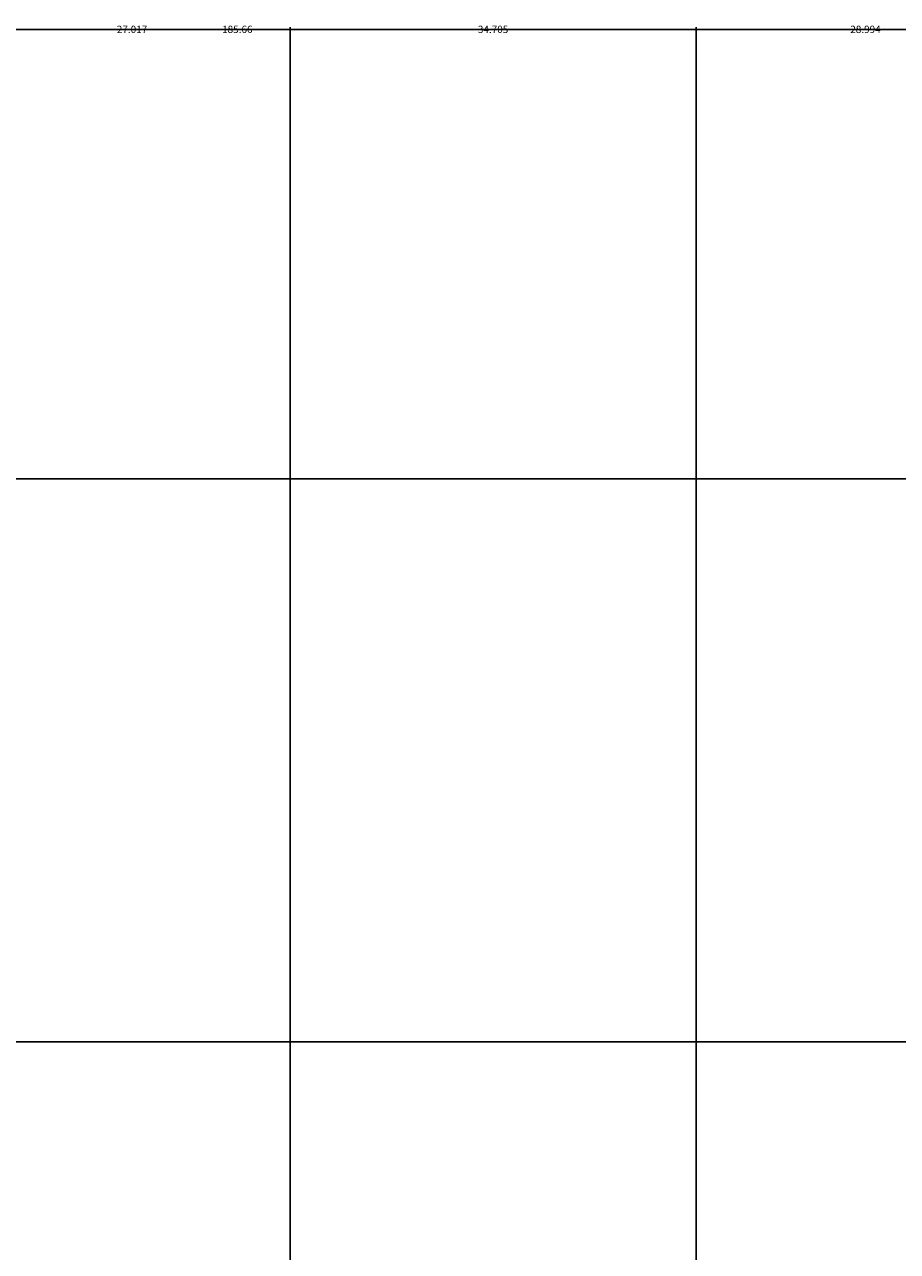
# Model space of a CAD drawing. Units: inches. Extents: x -13 to 809, y 112 to 656.
# Tile 32 of 55: x 182 to 257, y 551 to 656. Entities that reach past the tile are written whole.
import ezdxf

# ---------------------------------------------------------------- set-up
doc = ezdxf.new("R2010")
doc.units = ezdxf.units.IN
doc.header["$MEASUREMENT"] = 0
doc.layers.add('A-ANNO-DIMS', color=2, linetype='Continuous', lineweight=18)
doc.styles.get("Standard").update_dxf_attribs({"font": 'arial.ttf'})
doc.dimstyles.get("Standard").update_dxf_attribs({"dimtxt": 0.625, "dimasz": 0.18, "dimexe": 0.18, "dimexo": 0.0625, "dimgap": 0.09, "dimtad": 0, "dimtih": 1, "dimtoh": 1, "dimdec": 4, "dimzin": 0, "dimdsep": 46, "dimlunit": 4, "dimtxsty": 'Standard', "dimcen": 0.09, "dimadec": 0, "dimazin": 0, "dimtfac": 1, "dimtdec": 4, "dimtofl": 0, "dimtmove": 0, "dimatfit": 3, "dimfxl": 1, "dimtolj": 1, "dimtzin": 0, "dimarcsym": 0})

# ---------------------------------------------------------------- blocks, each defined once
blk = doc.blocks.new('*D23')
at = {"layer": 'A-ANNO-DIMS', "color": 0, "lineweight": -2, "transparency": 16777216}
for p, q in [((107.26, 510.58), (107.26, 655.96)), ((107.44, 655.78), (198.73, 655.78)), ((292.74, 655.78), (201.45, 655.78)), ((292.92, 569.3), (292.92, 655.96))]:
    blk.add_line(p, q, dxfattribs=at)
at = {"layer": 'A-ANNO-DIMS', "color": 0, "transparency": 16777216}
for points in [[(107.44, 655.81), (107.44, 655.75), (107.26, 655.78)], [(292.74, 655.81), (292.74, 655.75), (292.92, 655.78)]]:
    blk.add_solid(points, dxfattribs=at)
at = {"layer": 'Defpoints', "color": 0, "transparency": 16777216}
for p in [(292.92, 655.78), (292.92, 569.24), (107.26, 510.52)]:
    blk.add_point(p, dxfattribs=at)
at = {"layer": 'A-ANNO-DIMS', "color": 0, "transparency": 16777216, "insert": (200.09, 655.78), "char_height": 0.625, "attachment_point": 5}
blk.add_mtext('\\A1;185.66', dxfattribs=at)
blk = doc.blocks.new('*D36')
at = {"layer": 'A-ANNO-DIMS', "color": 0, "lineweight": -2, "transparency": 16777216}
for p, q in [((311.64, 569.24), (-12.1, 569.24)), ((-11.92, 569.06), (-11.92, 540.29)), ((-11.92, 510.7), (-11.92, 539.47)), ((107.2, 510.52), (-12.1, 510.52))]:
    blk.add_line(p, q, dxfattribs=at)
at = {"layer": 'A-ANNO-DIMS', "color": 0, "transparency": 16777216}
for points in [[(-11.95, 569.06), (-11.89, 569.06), (-11.92, 569.24)], [(-11.95, 510.7), (-11.89, 510.7), (-11.92, 510.52)]]:
    blk.add_solid(points, dxfattribs=at)
at = {"layer": 'Defpoints', "color": 0, "transparency": 16777216}
for p in [(-11.92, 569.24), (311.7, 569.24), (107.26, 510.52)]:
    blk.add_point(p, dxfattribs=at)
at = {"layer": 'A-ANNO-DIMS', "color": 0, "transparency": 16777216, "insert": (-11.92, 539.88), "char_height": 0.625, "attachment_point": 5}
blk.add_mtext('\\A1;58.72', dxfattribs=at)
blk = doc.blocks.new('*D37')
at = {"layer": 'A-ANNO-DIMS', "color": 0, "lineweight": -2, "transparency": 16777216}
for p, q in [((311.64, 617.37), (-12.1, 617.37)), ((-11.92, 617.19), (-11.92, 593.72)), ((-11.92, 569.42), (-11.92, 592.9)), ((311.64, 569.24), (-12.1, 569.24))]:
    blk.add_line(p, q, dxfattribs=at)
at = {"layer": 'A-ANNO-DIMS', "color": 0, "transparency": 16777216}
for points in [[(-11.95, 617.19), (-11.89, 617.19), (-11.92, 617.37)], [(-11.95, 569.42), (-11.89, 569.42), (-11.92, 569.24)]]:
    blk.add_solid(points, dxfattribs=at)
at = {"layer": 'Defpoints', "color": 0, "transparency": 16777216}
for p in [(-11.92, 617.37), (311.7, 617.37), (311.7, 569.24)]:
    blk.add_point(p, dxfattribs=at)
at = {"layer": 'A-ANNO-DIMS', "color": 0, "transparency": 16777216, "insert": (-11.92, 593.31), "char_height": 0.625, "attachment_point": 5}
blk.add_mtext('\\A1;48.13', dxfattribs=at)
blk = doc.blocks.new('*D98')
at = {"layer": 'A-ANNO-DIMS', "color": 0, "lineweight": -2, "transparency": 16777216}
for p, q in [((177.59, 452.63), (177.59, 655.96)), ((177.77, 655.78), (189.7, 655.78)), ((204.42, 655.78), (192.49, 655.78)), ((204.6, 452.63), (204.6, 655.96))]:
    blk.add_line(p, q, dxfattribs=at)
at = {"layer": 'A-ANNO-DIMS', "color": 0, "transparency": 16777216}
for points in [[(177.77, 655.81), (177.77, 655.75), (177.59, 655.78)], [(204.42, 655.81), (204.42, 655.75), (204.6, 655.78)]]:
    blk.add_solid(points, dxfattribs=at)
at = {"layer": 'Defpoints', "color": 0, "transparency": 16777216}
for p in [(204.6, 655.78), (177.59, 452.56), (204.6, 452.56)]:
    blk.add_point(p, dxfattribs=at)
at = {"layer": 'A-ANNO-DIMS', "color": 0, "transparency": 16777216, "insert": (191.09, 655.78), "char_height": 0.625, "attachment_point": 5}
blk.add_mtext('\\A1;27.017', dxfattribs=at)
blk = doc.blocks.new('*D99')
at = {"layer": 'A-ANNO-DIMS', "color": 0, "lineweight": -2, "transparency": 16777216}
for p, q in [((204.6, 452.63), (204.6, 655.96)), ((204.78, 655.78), (220.57, 655.78)), ((239.13, 655.78), (223.34, 655.78)), ((239.31, 452.63), (239.31, 655.96))]:
    blk.add_line(p, q, dxfattribs=at)
at = {"layer": 'A-ANNO-DIMS', "color": 0, "transparency": 16777216}
for points in [[(204.78, 655.81), (204.78, 655.75), (204.6, 655.78)], [(239.13, 655.81), (239.13, 655.75), (239.31, 655.78)]]:
    blk.add_solid(points, dxfattribs=at)
at = {"layer": 'Defpoints', "color": 0, "transparency": 16777216}
for p in [(239.31, 655.78), (204.6, 452.56), (239.31, 452.56)]:
    blk.add_point(p, dxfattribs=at)
at = {"layer": 'A-ANNO-DIMS', "color": 0, "transparency": 16777216, "insert": (221.96, 655.78), "char_height": 0.625, "attachment_point": 5}
blk.add_mtext('\\A1;34.705', dxfattribs=at)
blk = doc.blocks.new('*D100')
at = {"layer": 'A-ANNO-DIMS', "color": 0, "lineweight": -2, "transparency": 16777216}
for p, q in [((239.31, 452.63), (239.31, 655.96)), ((239.49, 655.78), (252.41, 655.78)), ((268.12, 655.78), (255.2, 655.78)), ((268.3, 452.63), (268.3, 655.96))]:
    blk.add_line(p, q, dxfattribs=at)
at = {"layer": 'A-ANNO-DIMS', "color": 0, "transparency": 16777216}
for points in [[(239.49, 655.81), (239.49, 655.75), (239.31, 655.78)], [(268.12, 655.81), (268.12, 655.75), (268.3, 655.78)]]:
    blk.add_solid(points, dxfattribs=at)
at = {"layer": 'Defpoints', "color": 0, "transparency": 16777216}
for p in [(268.3, 655.78), (239.31, 452.56), (268.3, 452.56)]:
    blk.add_point(p, dxfattribs=at)
at = {"layer": 'A-ANNO-DIMS', "color": 0, "transparency": 16777216, "insert": (253.8, 655.78), "char_height": 0.625, "attachment_point": 5}
blk.add_mtext('\\A1;28.994', dxfattribs=at)

msp = doc.modelspace()

# ---------------------------------------------------------------- dimensions: what is measured, and where the dimension line sits
at = {"layer": 'A-ANNO-DIMS'}
for base, p1, p2, override, picture, middle in [((292.923, 655.7828), (107.2588, 510.5199), (292.923, 569.2414), {"dimdec": 2, "dimlfac": 1, "dimrnd": 0, "dimzin": 0, "dimdsep": 46, "dimlunit": 2}, '*D23', (200.0909, 655.7828)), ((204.6029, 655.7828), (177.5857, 452.5629), (204.6029, 452.5629), {"dimdec": 3, "dimlfac": 1, "dimrnd": 0, "dimzin": 0, "dimdsep": 46, "dimlunit": 2}, '*D98', (191.0943, 655.7828)), ((239.3079, 655.7828), (204.6029, 452.5629), (239.3079, 452.5629), {"dimdec": 3, "dimlfac": 1, "dimrnd": 0, "dimzin": 0, "dimdsep": 46, "dimlunit": 2}, '*D99', (221.9554, 655.7828)), ((268.3019, 655.7828), (239.3079, 452.5629), (268.3019, 452.5629), {"dimdec": 3, "dimlfac": 1, "dimrnd": 0, "dimzin": 0, "dimdsep": 46, "dimlunit": 2}, '*D100', (253.8049, 655.7828))]:
    dim = msp.add_linear_dim(base=base, p1=p1, p2=p2, dimstyle='Standard', override=override, dxfattribs=at)
    dim.commit()
    dim.dimension.update_dxf_attribs({"geometry": picture, "text_midpoint": middle})
for base, p1, p2, picture, middle in [((-11.9191, 617.3708), (311.6991, 569.2414), (311.6991, 617.3708), '*D37', (-11.9191, 593.3061)), ((-11.9191, 569.2414), (107.2588, 510.5199), (311.6991, 569.2414), '*D36', (-11.9191, 539.8806))]:
    dim = msp.add_linear_dim(base=base, p1=p1, p2=p2, angle=90, dimstyle='Standard', override={"dimdec": 2, "dimlfac": 1, "dimrnd": 0, "dimzin": 0, "dimdsep": 46, "dimlunit": 2}, dxfattribs=at)
    dim.commit()
    dim.dimension.update_dxf_attribs({"geometry": picture, "text_midpoint": middle})

doc.saveas('drawing.dxf')
